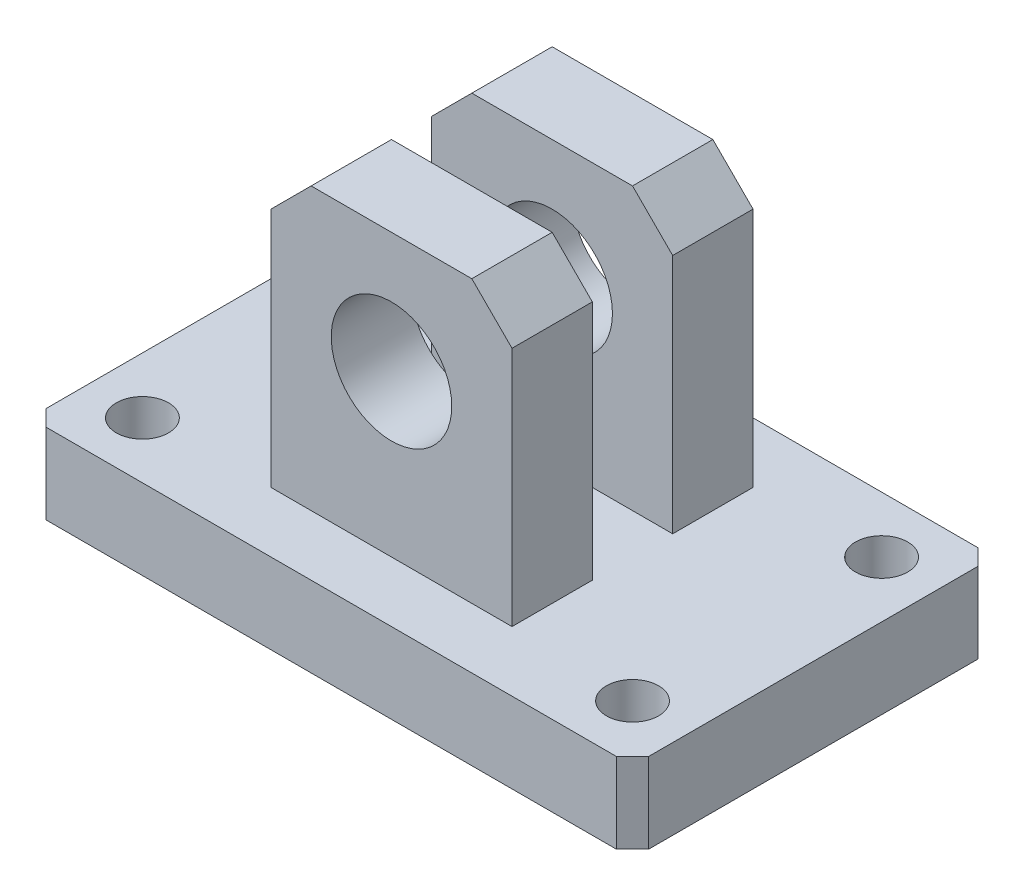
ISO-10303-21;
HEADER;
FILE_DESCRIPTION(('STEP AP214'),'2;1');
FILE_NAME('part.step','',(''),(''),'','','');
FILE_SCHEMA(('AUTOMOTIVE_DESIGN { 1 0 10303 214 1 1 1 1 }'));
ENDSEC;
DATA;
#1=APPLICATION_CONTEXT('core data for automotive mechanical design processes');
#2=APPLICATION_PROTOCOL_DEFINITION('international standard','automotive_design',2000,#1);
#3=PRODUCT_CONTEXT('',#1,'mechanical');
#4=PRODUCT('Part','Part','',(#3));
#5=PRODUCT_RELATED_PRODUCT_CATEGORY('part','',(#4));
#6=PRODUCT_DEFINITION_FORMATION('','',#4);
#7=PRODUCT_DEFINITION_CONTEXT('part definition',#1,'design');
#8=PRODUCT_DEFINITION('design','',#6,#7);
#9=PRODUCT_DEFINITION_SHAPE('','',#8);
#10=(LENGTH_UNIT() NAMED_UNIT(*) SI_UNIT(.MILLI.,.METRE.));
#11=(NAMED_UNIT(*) PLANE_ANGLE_UNIT() SI_UNIT($,.RADIAN.));
#12=(NAMED_UNIT(*) SI_UNIT($,.STERADIAN.) SOLID_ANGLE_UNIT());
#13=UNCERTAINTY_MEASURE_WITH_UNIT(LENGTH_MEASURE(1.E-05),#10,'distance_accuracy_value','');
#14=(GEOMETRIC_REPRESENTATION_CONTEXT(3) GLOBAL_UNCERTAINTY_ASSIGNED_CONTEXT((#13)) GLOBAL_UNIT_ASSIGNED_CONTEXT((#10,
#11,#12)) REPRESENTATION_CONTEXT('',''));
#15=CARTESIAN_POINT('',(0.,0.,0.));
#16=DIRECTION('',(0.,0.,1.));
#17=DIRECTION('',(1.,0.,0.));
#18=AXIS2_PLACEMENT_3D('',#15,#16,#17);
#19=CARTESIAN_POINT('',(0.,10.,0.));
#20=DIRECTION('',(0.,1.,0.));
#21=DIRECTION('',(0.,0.,1.));
#22=AXIS2_PLACEMENT_3D('',#19,#20,#21);
#23=PLANE('',#22);
#24=CARTESIAN_POINT('',(30.5,10.,-15.5));
#25=DIRECTION('',(0.,-1.,0.));
#26=DIRECTION('',(0.,0.,1.));
#27=AXIS2_PLACEMENT_3D('',#24,#25,#26);
#28=CIRCLE('',#27,3.25);
#29=CARTESIAN_POINT('',(30.5,10.,-12.25));
#30=VERTEX_POINT('',#29);
#31=EDGE_CURVE('E566',#30,#30,#28,.T.);
#32=ORIENTED_EDGE('',*,*,#31,.T.);
#33=EDGE_LOOP('',(#32));
#34=FACE_BOUND('',#33,.T.);
#35=CARTESIAN_POINT('',(30.5,10.,15.5));
#36=DIRECTION('',(0.,1.,0.));
#37=DIRECTION('',(0.,0.,-1.));
#38=AXIS2_PLACEMENT_3D('',#35,#36,#37);
#39=CIRCLE('',#38,3.25);
#40=CARTESIAN_POINT('',(30.5,10.,12.25));
#41=VERTEX_POINT('',#40);
#42=EDGE_CURVE('E576',#41,#41,#39,.T.);
#43=ORIENTED_EDGE('',*,*,#42,.F.);
#44=EDGE_LOOP('',(#43));
#45=FACE_BOUND('',#44,.T.);
#46=CARTESIAN_POINT('',(-30.5,10.,15.5));
#47=DIRECTION('',(0.,-1.,0.));
#48=DIRECTION('',(0.,0.,-1.));
#49=AXIS2_PLACEMENT_3D('',#46,#47,#48);
#50=CIRCLE('',#49,3.25);
#51=CARTESIAN_POINT('',(-30.5,10.,12.25));
#52=VERTEX_POINT('',#51);
#53=EDGE_CURVE('E581',#52,#52,#50,.T.);
#54=ORIENTED_EDGE('',*,*,#53,.T.);
#55=EDGE_LOOP('',(#54));
#56=FACE_BOUND('',#55,.T.);
#57=CARTESIAN_POINT('',(-30.5,10.,-15.5));
#58=DIRECTION('',(0.,1.,0.));
#59=DIRECTION('',(0.,0.,1.));
#60=AXIS2_PLACEMENT_3D('',#57,#58,#59);
#61=CIRCLE('',#60,3.25);
#62=CARTESIAN_POINT('',(-30.5,10.,-12.25));
#63=VERTEX_POINT('',#62);
#64=EDGE_CURVE('E589',#63,#63,#61,.T.);
#65=ORIENTED_EDGE('',*,*,#64,.F.);
#66=EDGE_LOOP('',(#65));
#67=FACE_BOUND('',#66,.T.);
#68=DIRECTION('',(0.,0.,1.));
#69=VECTOR('',#68,1.);
#70=CARTESIAN_POINT('',(15.,10.,-15.));
#71=LINE('',#70,#69);
#72=CARTESIAN_POINT('',(15.,10.,-15.));
#73=VERTEX_POINT('',#72);
#74=CARTESIAN_POINT('',(15.,10.,-5.00000000000001));
#75=VERTEX_POINT('',#74);
#76=EDGE_CURVE('E188',#73,#75,#71,.T.);
#77=ORIENTED_EDGE('',*,*,#76,.T.);
#78=DIRECTION('',(-1.,0.,0.));
#79=VECTOR('',#78,1.);
#80=CARTESIAN_POINT('',(-15.,10.,-5.00000000000001));
#81=LINE('',#80,#79);
#82=CARTESIAN_POINT('',(-15.,10.,-5.00000000000001));
#83=VERTEX_POINT('',#82);
#84=EDGE_CURVE('E196',#75,#83,#81,.T.);
#85=ORIENTED_EDGE('',*,*,#84,.T.);
#86=DIRECTION('',(0.,0.,-1.));
#87=VECTOR('',#86,1.);
#88=CARTESIAN_POINT('',(-15.,10.,-15.));
#89=LINE('',#88,#87);
#90=CARTESIAN_POINT('',(-15.,10.,-15.));
#91=VERTEX_POINT('',#90);
#92=EDGE_CURVE('E208',#83,#91,#89,.T.);
#93=ORIENTED_EDGE('',*,*,#92,.T.);
#94=DIRECTION('',(1.,0.,0.));
#95=VECTOR('',#94,1.);
#96=CARTESIAN_POINT('',(-15.,10.,-15.));
#97=LINE('',#96,#95);
#98=EDGE_CURVE('E203',#91,#73,#97,.T.);
#99=ORIENTED_EDGE('',*,*,#98,.T.);
#100=EDGE_LOOP('',(#77,#85,#93,#99));
#101=FACE_BOUND('',#100,.T.);
#102=DIRECTION('',(0.,0.,1.));
#103=VECTOR('',#102,1.);
#104=CARTESIAN_POINT('',(-37.5,10.,22.5));
#105=LINE('',#104,#103);
#106=CARTESIAN_POINT('',(-37.5,10.,-20.5));
#107=VERTEX_POINT('',#106);
#108=CARTESIAN_POINT('',(-37.5,10.,20.5));
#109=VERTEX_POINT('',#108);
#110=EDGE_CURVE('E250',#107,#109,#105,.T.);
#111=ORIENTED_EDGE('',*,*,#110,.T.);
#112=DIRECTION('',(-0.707106781186545,0.,-0.70710678118655));
#113=VECTOR('',#112,1.);
#114=CARTESIAN_POINT('',(-29.0000000000001,10.,28.9999999999999));
#115=LINE('',#114,#113);
#116=CARTESIAN_POINT('',(-35.5,10.,22.5));
#117=VERTEX_POINT('',#116);
#118=EDGE_CURVE('E322',#109,#117,#115,.F.);
#119=ORIENTED_EDGE('',*,*,#118,.T.);
#120=DIRECTION('',(1.,0.,0.));
#121=VECTOR('',#120,1.);
#122=CARTESIAN_POINT('',(37.5,10.,22.5));
#123=LINE('',#122,#121);
#124=CARTESIAN_POINT('',(35.5,10.,22.5));
#125=VERTEX_POINT('',#124);
#126=EDGE_CURVE('E247',#117,#125,#123,.T.);
#127=ORIENTED_EDGE('',*,*,#126,.T.);
#128=DIRECTION('',(-0.70710678118655,0.,0.707106781186545));
#129=VECTOR('',#128,1.);
#130=CARTESIAN_POINT('',(28.9999999999999,10.,29.0000000000001));
#131=LINE('',#130,#129);
#132=CARTESIAN_POINT('',(37.5,10.,20.5));
#133=VERTEX_POINT('',#132);
#134=EDGE_CURVE('E317',#125,#133,#131,.F.);
#135=ORIENTED_EDGE('',*,*,#134,.T.);
#136=DIRECTION('',(0.,0.,-1.));
#137=VECTOR('',#136,1.);
#138=CARTESIAN_POINT('',(37.5,10.,22.5));
#139=LINE('',#138,#137);
#140=CARTESIAN_POINT('',(37.5,10.,-20.5));
#141=VERTEX_POINT('',#140);
#142=EDGE_CURVE('E255',#133,#141,#139,.T.);
#143=ORIENTED_EDGE('',*,*,#142,.T.);
#144=DIRECTION('',(0.707106781186545,0.,0.70710678118655));
#145=VECTOR('',#144,1.);
#146=CARTESIAN_POINT('',(29.0000000000001,10.,-28.9999999999999));
#147=LINE('',#146,#145);
#148=CARTESIAN_POINT('',(35.5,10.,-22.5));
#149=VERTEX_POINT('',#148);
#150=EDGE_CURVE('E61',#141,#149,#147,.F.);
#151=ORIENTED_EDGE('',*,*,#150,.T.);
#152=DIRECTION('',(-1.,0.,0.));
#153=VECTOR('',#152,1.);
#154=CARTESIAN_POINT('',(37.5,10.,-22.5));
#155=LINE('',#154,#153);
#156=CARTESIAN_POINT('',(-35.5,10.,-22.5));
#157=VERTEX_POINT('',#156);
#158=EDGE_CURVE('E258',#149,#157,#155,.T.);
#159=ORIENTED_EDGE('',*,*,#158,.T.);
#160=DIRECTION('',(0.70710678118655,0.,-0.707106781186545));
#161=VECTOR('',#160,1.);
#162=CARTESIAN_POINT('',(-28.9999999999999,10.,-29.0000000000001));
#163=LINE('',#162,#161);
#164=EDGE_CURVE('E325',#157,#107,#163,.F.);
#165=ORIENTED_EDGE('',*,*,#164,.T.);
#166=EDGE_LOOP('',(#111,#119,#127,#135,#143,#151,#159,#165));
#167=FACE_BOUND('',#166,.T.);
#168=DIRECTION('',(-1.,0.,0.));
#169=VECTOR('',#168,1.);
#170=CARTESIAN_POINT('',(-15.,10.,5.00000000000001));
#171=LINE('',#170,#169);
#172=CARTESIAN_POINT('',(15.,10.,5.00000000000001));
#173=VERTEX_POINT('',#172);
#174=CARTESIAN_POINT('',(-15.,10.,5.00000000000001));
#175=VERTEX_POINT('',#174);
#176=EDGE_CURVE('E233',#173,#175,#171,.T.);
#177=ORIENTED_EDGE('',*,*,#176,.F.);
#178=DIRECTION('',(0.,0.,-1.));
#179=VECTOR('',#178,1.);
#180=CARTESIAN_POINT('',(15.,10.,15.));
#181=LINE('',#180,#179);
#182=CARTESIAN_POINT('',(15.,10.,15.));
#183=VERTEX_POINT('',#182);
#184=EDGE_CURVE('E219',#183,#173,#181,.T.);
#185=ORIENTED_EDGE('',*,*,#184,.F.);
#186=DIRECTION('',(1.,0.,0.));
#187=VECTOR('',#186,1.);
#188=CARTESIAN_POINT('',(-15.,10.,15.));
#189=LINE('',#188,#187);
#190=CARTESIAN_POINT('',(-15.,10.,15.));
#191=VERTEX_POINT('',#190);
#192=EDGE_CURVE('E223',#191,#183,#189,.T.);
#193=ORIENTED_EDGE('',*,*,#192,.F.);
#194=DIRECTION('',(0.,0.,1.));
#195=VECTOR('',#194,1.);
#196=CARTESIAN_POINT('',(-15.,10.,15.));
#197=LINE('',#196,#195);
#198=EDGE_CURVE('E234',#175,#191,#197,.T.);
#199=ORIENTED_EDGE('',*,*,#198,.F.);
#200=EDGE_LOOP('',(#177,#185,#193,#199));
#201=FACE_BOUND('',#200,.T.);
#202=ADVANCED_FACE('F41',(#34,#45,#56,#67,#101,#167,#201),#23,.T.);
#203=CARTESIAN_POINT('',(-37.5,10.,22.5));
#204=DIRECTION('',(1.,0.,0.));
#205=DIRECTION('',(0.,0.,-1.));
#206=AXIS2_PLACEMENT_3D('',#203,#204,#205);
#207=PLANE('',#206);
#208=DIRECTION('',(0.,0.,1.));
#209=VECTOR('',#208,1.);
#210=CARTESIAN_POINT('',(-37.5,0.,22.5));
#211=LINE('',#210,#209);
#212=CARTESIAN_POINT('',(-37.5,0.,-20.5));
#213=VERTEX_POINT('',#212);
#214=CARTESIAN_POINT('',(-37.5,0.,20.5));
#215=VERTEX_POINT('',#214);
#216=EDGE_CURVE('E248',#213,#215,#211,.T.);
#217=ORIENTED_EDGE('',*,*,#216,.T.);
#218=DIRECTION('',(0.,1.,0.));
#219=VECTOR('',#218,1.);
#220=CARTESIAN_POINT('',(-37.5,10.,20.5));
#221=LINE('',#220,#219);
#222=EDGE_CURVE('E320',#215,#109,#221,.T.);
#223=ORIENTED_EDGE('',*,*,#222,.T.);
#224=ORIENTED_EDGE('',*,*,#110,.F.);
#225=DIRECTION('',(0.,-1.,0.));
#226=VECTOR('',#225,1.);
#227=CARTESIAN_POINT('',(-37.5,10.,-20.5));
#228=LINE('',#227,#226);
#229=EDGE_CURVE('E314',#107,#213,#228,.T.);
#230=ORIENTED_EDGE('',*,*,#229,.T.);
#231=EDGE_LOOP('',(#217,#223,#224,#230));
#232=FACE_BOUND('',#231,.T.);
#233=ADVANCED_FACE('F351',(#232),#207,.F.);
#234=CARTESIAN_POINT('',(37.5,10.,22.5));
#235=DIRECTION('',(0.,0.,-1.));
#236=DIRECTION('',(-1.,0.,0.));
#237=AXIS2_PLACEMENT_3D('',#234,#235,#236);
#238=PLANE('',#237);
#239=ORIENTED_EDGE('',*,*,#126,.F.);
#240=DIRECTION('',(0.,-1.,0.));
#241=VECTOR('',#240,1.);
#242=CARTESIAN_POINT('',(-35.5,10.,22.5));
#243=LINE('',#242,#241);
#244=CARTESIAN_POINT('',(-35.5,0.,22.5));
#245=VERTEX_POINT('',#244);
#246=EDGE_CURVE('E301',#117,#245,#243,.T.);
#247=ORIENTED_EDGE('',*,*,#246,.T.);
#248=DIRECTION('',(1.,0.,0.));
#249=VECTOR('',#248,1.);
#250=CARTESIAN_POINT('',(37.5,0.,22.5));
#251=LINE('',#250,#249);
#252=CARTESIAN_POINT('',(35.5,0.,22.5));
#253=VERTEX_POINT('',#252);
#254=EDGE_CURVE('E261',#245,#253,#251,.T.);
#255=ORIENTED_EDGE('',*,*,#254,.T.);
#256=DIRECTION('',(0.,1.,0.));
#257=VECTOR('',#256,1.);
#258=CARTESIAN_POINT('',(35.5,10.,22.5));
#259=LINE('',#258,#257);
#260=EDGE_CURVE('E303',#253,#125,#259,.T.);
#261=ORIENTED_EDGE('',*,*,#260,.T.);
#262=EDGE_LOOP('',(#239,#247,#255,#261));
#263=FACE_BOUND('',#262,.T.);
#264=ADVANCED_FACE('F361',(#263),#238,.F.);
#265=CARTESIAN_POINT('',(37.5,10.,22.5));
#266=DIRECTION('',(-1.,0.,0.));
#267=DIRECTION('',(0.,0.,1.));
#268=AXIS2_PLACEMENT_3D('',#265,#266,#267);
#269=PLANE('',#268);
#270=DIRECTION('',(0.,0.,-1.));
#271=VECTOR('',#270,1.);
#272=CARTESIAN_POINT('',(37.5,0.,22.5));
#273=LINE('',#272,#271);
#274=CARTESIAN_POINT('',(37.5,0.,20.5));
#275=VERTEX_POINT('',#274);
#276=CARTESIAN_POINT('',(37.5,0.,-20.5));
#277=VERTEX_POINT('',#276);
#278=EDGE_CURVE('E262',#275,#277,#273,.T.);
#279=ORIENTED_EDGE('',*,*,#278,.T.);
#280=DIRECTION('',(0.,1.,0.));
#281=VECTOR('',#280,1.);
#282=CARTESIAN_POINT('',(37.5,10.,-20.5));
#283=LINE('',#282,#281);
#284=EDGE_CURVE('E11',#277,#141,#283,.T.);
#285=ORIENTED_EDGE('',*,*,#284,.T.);
#286=ORIENTED_EDGE('',*,*,#142,.F.);
#287=DIRECTION('',(0.,-1.,0.));
#288=VECTOR('',#287,1.);
#289=CARTESIAN_POINT('',(37.5,10.,20.5));
#290=LINE('',#289,#288);
#291=EDGE_CURVE('E51',#133,#275,#290,.T.);
#292=ORIENTED_EDGE('',*,*,#291,.T.);
#293=EDGE_LOOP('',(#279,#285,#286,#292));
#294=FACE_BOUND('',#293,.T.);
#295=ADVANCED_FACE('F333',(#294),#269,.F.);
#296=CARTESIAN_POINT('',(37.5,10.,-22.5));
#297=DIRECTION('',(0.,0.,1.));
#298=DIRECTION('',(1.,0.,0.));
#299=AXIS2_PLACEMENT_3D('',#296,#297,#298);
#300=PLANE('',#299);
#301=DIRECTION('',(-1.,0.,0.));
#302=VECTOR('',#301,1.);
#303=CARTESIAN_POINT('',(37.5,0.,-22.5));
#304=LINE('',#303,#302);
#305=CARTESIAN_POINT('',(35.5,0.,-22.5));
#306=VERTEX_POINT('',#305);
#307=CARTESIAN_POINT('',(-35.5,0.,-22.5));
#308=VERTEX_POINT('',#307);
#309=EDGE_CURVE('E253',#306,#308,#304,.T.);
#310=ORIENTED_EDGE('',*,*,#309,.T.);
#311=DIRECTION('',(0.,1.,0.));
#312=VECTOR('',#311,1.);
#313=CARTESIAN_POINT('',(-35.5,10.,-22.5));
#314=LINE('',#313,#312);
#315=EDGE_CURVE('E59',#308,#157,#314,.T.);
#316=ORIENTED_EDGE('',*,*,#315,.T.);
#317=ORIENTED_EDGE('',*,*,#158,.F.);
#318=DIRECTION('',(0.,-1.,0.));
#319=VECTOR('',#318,1.);
#320=CARTESIAN_POINT('',(35.5,10.,-22.5));
#321=LINE('',#320,#319);
#322=EDGE_CURVE('E326',#149,#306,#321,.T.);
#323=ORIENTED_EDGE('',*,*,#322,.T.);
#324=EDGE_LOOP('',(#310,#316,#317,#323));
#325=FACE_BOUND('',#324,.T.);
#326=ADVANCED_FACE('F347',(#325),#300,.F.);
#327=CARTESIAN_POINT('',(0.,0.,0.));
#328=DIRECTION('',(0.,1.,0.));
#329=DIRECTION('',(0.,0.,1.));
#330=AXIS2_PLACEMENT_3D('',#327,#328,#329);
#331=PLANE('',#330);
#332=CARTESIAN_POINT('',(30.5,0.,-15.5));
#333=DIRECTION('',(0.,-1.,0.));
#334=DIRECTION('',(0.,0.,1.));
#335=AXIS2_PLACEMENT_3D('',#332,#333,#334);
#336=CIRCLE('',#335,3.25);
#337=CARTESIAN_POINT('',(30.5,0.,-12.25));
#338=VERTEX_POINT('',#337);
#339=EDGE_CURVE('E573',#338,#338,#336,.T.);
#340=ORIENTED_EDGE('',*,*,#339,.F.);
#341=EDGE_LOOP('',(#340));
#342=FACE_BOUND('',#341,.T.);
#343=CARTESIAN_POINT('',(30.5,0.,15.5));
#344=DIRECTION('',(0.,1.,0.));
#345=DIRECTION('',(0.,0.,-1.));
#346=AXIS2_PLACEMENT_3D('',#343,#344,#345);
#347=CIRCLE('',#346,3.25);
#348=CARTESIAN_POINT('',(30.5,0.,12.25));
#349=VERTEX_POINT('',#348);
#350=EDGE_CURVE('E577',#349,#349,#347,.T.);
#351=ORIENTED_EDGE('',*,*,#350,.T.);
#352=EDGE_LOOP('',(#351));
#353=FACE_BOUND('',#352,.T.);
#354=CARTESIAN_POINT('',(-30.5,0.,15.5));
#355=DIRECTION('',(0.,-1.,0.));
#356=DIRECTION('',(0.,0.,-1.));
#357=AXIS2_PLACEMENT_3D('',#354,#355,#356);
#358=CIRCLE('',#357,3.25);
#359=CARTESIAN_POINT('',(-30.5,0.,12.25));
#360=VERTEX_POINT('',#359);
#361=EDGE_CURVE('E588',#360,#360,#358,.T.);
#362=ORIENTED_EDGE('',*,*,#361,.F.);
#363=EDGE_LOOP('',(#362));
#364=FACE_BOUND('',#363,.T.);
#365=CARTESIAN_POINT('',(-30.5,0.,-15.5));
#366=DIRECTION('',(0.,1.,0.));
#367=DIRECTION('',(0.,0.,1.));
#368=AXIS2_PLACEMENT_3D('',#365,#366,#367);
#369=CIRCLE('',#368,3.25);
#370=CARTESIAN_POINT('',(-30.5,0.,-12.25));
#371=VERTEX_POINT('',#370);
#372=EDGE_CURVE('E205',#371,#371,#369,.T.);
#373=ORIENTED_EDGE('',*,*,#372,.T.);
#374=EDGE_LOOP('',(#373));
#375=FACE_BOUND('',#374,.T.);
#376=ORIENTED_EDGE('',*,*,#254,.F.);
#377=DIRECTION('',(0.707106781186545,0.,0.70710678118655));
#378=VECTOR('',#377,1.);
#379=CARTESIAN_POINT('',(-35.5,0.,22.5));
#380=LINE('',#379,#378);
#381=EDGE_CURVE('E315',#245,#215,#380,.F.);
#382=ORIENTED_EDGE('',*,*,#381,.T.);
#383=ORIENTED_EDGE('',*,*,#216,.F.);
#384=DIRECTION('',(-0.70710678118655,0.,0.707106781186545));
#385=VECTOR('',#384,1.);
#386=CARTESIAN_POINT('',(-37.5,0.,-20.5));
#387=LINE('',#386,#385);
#388=EDGE_CURVE('E309',#213,#308,#387,.F.);
#389=ORIENTED_EDGE('',*,*,#388,.T.);
#390=ORIENTED_EDGE('',*,*,#309,.F.);
#391=DIRECTION('',(-0.707106781186545,0.,-0.70710678118655));
#392=VECTOR('',#391,1.);
#393=CARTESIAN_POINT('',(35.5,0.,-22.5));
#394=LINE('',#393,#392);
#395=EDGE_CURVE('E306',#306,#277,#394,.F.);
#396=ORIENTED_EDGE('',*,*,#395,.T.);
#397=ORIENTED_EDGE('',*,*,#278,.F.);
#398=DIRECTION('',(0.70710678118655,0.,-0.707106781186545));
#399=VECTOR('',#398,1.);
#400=CARTESIAN_POINT('',(37.5,0.,20.5));
#401=LINE('',#400,#399);
#402=EDGE_CURVE('E308',#275,#253,#401,.F.);
#403=ORIENTED_EDGE('',*,*,#402,.T.);
#404=EDGE_LOOP('',(#376,#382,#383,#389,#390,#396,#397,#403));
#405=FACE_BOUND('',#404,.T.);
#406=ADVANCED_FACE('F343',(#342,#353,#364,#375,#405),#331,.F.);
#407=CARTESIAN_POINT('',(15.,45.,15.));
#408=DIRECTION('',(-1.,0.,0.));
#409=DIRECTION('',(0.,0.,1.));
#410=AXIS2_PLACEMENT_3D('',#407,#408,#409);
#411=PLANE('',#410);
#412=DIRECTION('',(0.,-1.,0.));
#413=VECTOR('',#412,1.);
#414=CARTESIAN_POINT('',(15.,45.,5.00000000000001));
#415=LINE('',#414,#413);
#416=CARTESIAN_POINT('',(15.,40.,5.00000000000001));
#417=VERTEX_POINT('',#416);
#418=EDGE_CURVE('E245',#417,#173,#415,.T.);
#419=ORIENTED_EDGE('',*,*,#418,.F.);
#420=DIRECTION('',(0.,0.,1.));
#421=VECTOR('',#420,1.);
#422=CARTESIAN_POINT('',(15.,40.,15.));
#423=LINE('',#422,#421);
#424=CARTESIAN_POINT('',(15.,40.,15.));
#425=VERTEX_POINT('',#424);
#426=EDGE_CURVE('E300',#417,#425,#423,.T.);
#427=ORIENTED_EDGE('',*,*,#426,.T.);
#428=DIRECTION('',(0.,-1.,0.));
#429=VECTOR('',#428,1.);
#430=CARTESIAN_POINT('',(15.,45.,15.));
#431=LINE('',#430,#429);
#432=EDGE_CURVE('E227',#425,#183,#431,.T.);
#433=ORIENTED_EDGE('',*,*,#432,.T.);
#434=ORIENTED_EDGE('',*,*,#184,.T.);
#435=EDGE_LOOP('',(#419,#427,#433,#434));
#436=FACE_BOUND('',#435,.T.);
#437=ADVANCED_FACE('F390',(#436),#411,.F.);
#438=CARTESIAN_POINT('',(-15.,45.,5.00000000000001));
#439=DIRECTION('',(0.,0.,1.));
#440=DIRECTION('',(1.,0.,0.));
#441=AXIS2_PLACEMENT_3D('',#438,#439,#440);
#442=PLANE('',#441);
#443=CARTESIAN_POINT('',(0.,30.,5.00000000000001));
#444=DIRECTION('',(0.,0.,1.));
#445=DIRECTION('',(1.,0.,0.));
#446=AXIS2_PLACEMENT_3D('',#443,#444,#445);
#447=CIRCLE('',#446,7.5);
#448=CARTESIAN_POINT('',(7.5,30.,5.00000000000001));
#449=VERTEX_POINT('',#448);
#450=EDGE_CURVE('E549',#449,#449,#447,.T.);
#451=ORIENTED_EDGE('',*,*,#450,.T.);
#452=EDGE_LOOP('',(#451));
#453=FACE_BOUND('',#452,.T.);
#454=DIRECTION('',(0.,-1.,0.));
#455=VECTOR('',#454,1.);
#456=CARTESIAN_POINT('',(-15.,45.,5.00000000000001));
#457=LINE('',#456,#455);
#458=CARTESIAN_POINT('',(-15.,40.,5.00000000000001));
#459=VERTEX_POINT('',#458);
#460=EDGE_CURVE('E244',#459,#175,#457,.T.);
#461=ORIENTED_EDGE('',*,*,#460,.F.);
#462=DIRECTION('',(-0.707106781186547,-0.707106781186549,0.));
#463=VECTOR('',#462,1.);
#464=CARTESIAN_POINT('',(-9.99999999999999,45.,5.00000000000001));
#465=LINE('',#464,#463);
#466=CARTESIAN_POINT('',(-9.99999999999999,45.,5.00000000000001));
#467=VERTEX_POINT('',#466);
#468=EDGE_CURVE('E283',#459,#467,#465,.F.);
#469=ORIENTED_EDGE('',*,*,#468,.T.);
#470=DIRECTION('',(-1.,0.,0.));
#471=VECTOR('',#470,1.);
#472=CARTESIAN_POINT('',(-15.,45.,5.00000000000001));
#473=LINE('',#472,#471);
#474=CARTESIAN_POINT('',(10.,45.,5.00000000000001));
#475=VERTEX_POINT('',#474);
#476=EDGE_CURVE('E222',#475,#467,#473,.T.);
#477=ORIENTED_EDGE('',*,*,#476,.F.);
#478=DIRECTION('',(-0.707106781186547,0.707106781186549,0.));
#479=VECTOR('',#478,1.);
#480=CARTESIAN_POINT('',(10.,45.,5.00000000000001));
#481=LINE('',#480,#479);
#482=EDGE_CURVE('E276',#475,#417,#481,.F.);
#483=ORIENTED_EDGE('',*,*,#482,.T.);
#484=ORIENTED_EDGE('',*,*,#418,.T.);
#485=ORIENTED_EDGE('',*,*,#176,.T.);
#486=EDGE_LOOP('',(#461,#469,#477,#483,#484,#485));
#487=FACE_BOUND('',#486,.T.);
#488=ADVANCED_FACE('F539',(#453,#487),#442,.F.);
#489=CARTESIAN_POINT('',(-15.,45.,15.));
#490=DIRECTION('',(1.,0.,0.));
#491=DIRECTION('',(0.,0.,-1.));
#492=AXIS2_PLACEMENT_3D('',#489,#490,#491);
#493=PLANE('',#492);
#494=DIRECTION('',(0.,-1.,0.));
#495=VECTOR('',#494,1.);
#496=CARTESIAN_POINT('',(-15.,45.,15.));
#497=LINE('',#496,#495);
#498=CARTESIAN_POINT('',(-15.,40.,15.));
#499=VERTEX_POINT('',#498);
#500=EDGE_CURVE('E238',#499,#191,#497,.T.);
#501=ORIENTED_EDGE('',*,*,#500,.F.);
#502=DIRECTION('',(0.,0.,-1.));
#503=VECTOR('',#502,1.);
#504=CARTESIAN_POINT('',(-15.,40.,15.));
#505=LINE('',#504,#503);
#506=EDGE_CURVE('E280',#499,#459,#505,.T.);
#507=ORIENTED_EDGE('',*,*,#506,.T.);
#508=ORIENTED_EDGE('',*,*,#460,.T.);
#509=ORIENTED_EDGE('',*,*,#198,.T.);
#510=EDGE_LOOP('',(#501,#507,#508,#509));
#511=FACE_BOUND('',#510,.T.);
#512=ADVANCED_FACE('F540',(#511),#493,.F.);
#513=CARTESIAN_POINT('',(-15.,45.,15.));
#514=DIRECTION('',(0.,0.,-1.));
#515=DIRECTION('',(-1.,0.,0.));
#516=AXIS2_PLACEMENT_3D('',#513,#514,#515);
#517=PLANE('',#516);
#518=CARTESIAN_POINT('',(0.,30.,15.));
#519=DIRECTION('',(0.,0.,1.));
#520=DIRECTION('',(1.,0.,0.));
#521=AXIS2_PLACEMENT_3D('',#518,#519,#520);
#522=CIRCLE('',#521,7.5);
#523=CARTESIAN_POINT('',(7.5,30.,15.));
#524=VERTEX_POINT('',#523);
#525=EDGE_CURVE('E625',#524,#524,#522,.T.);
#526=ORIENTED_EDGE('',*,*,#525,.F.);
#527=EDGE_LOOP('',(#526));
#528=FACE_BOUND('',#527,.T.);
#529=DIRECTION('',(1.,0.,0.));
#530=VECTOR('',#529,1.);
#531=CARTESIAN_POINT('',(-15.,45.,15.));
#532=LINE('',#531,#530);
#533=CARTESIAN_POINT('',(-9.99999999999999,45.,15.));
#534=VERTEX_POINT('',#533);
#535=CARTESIAN_POINT('',(10.,45.,15.));
#536=VERTEX_POINT('',#535);
#537=EDGE_CURVE('E221',#534,#536,#532,.T.);
#538=ORIENTED_EDGE('',*,*,#537,.F.);
#539=DIRECTION('',(0.707106781186547,0.707106781186549,0.));
#540=VECTOR('',#539,1.);
#541=CARTESIAN_POINT('',(-9.99999999999999,45.,15.));
#542=LINE('',#541,#540);
#543=EDGE_CURVE('E274',#534,#499,#542,.F.);
#544=ORIENTED_EDGE('',*,*,#543,.T.);
#545=ORIENTED_EDGE('',*,*,#500,.T.);
#546=ORIENTED_EDGE('',*,*,#192,.T.);
#547=ORIENTED_EDGE('',*,*,#432,.F.);
#548=DIRECTION('',(0.707106781186547,-0.707106781186549,0.));
#549=VECTOR('',#548,1.);
#550=CARTESIAN_POINT('',(10.,45.,15.));
#551=LINE('',#550,#549);
#552=EDGE_CURVE('E272',#425,#536,#551,.F.);
#553=ORIENTED_EDGE('',*,*,#552,.T.);
#554=EDGE_LOOP('',(#538,#544,#545,#546,#547,#553));
#555=FACE_BOUND('',#554,.T.);
#556=ADVANCED_FACE('F531',(#528,#555),#517,.F.);
#557=CARTESIAN_POINT('',(0.,45.,0.));
#558=DIRECTION('',(0.,-1.,0.));
#559=DIRECTION('',(0.,0.,-1.));
#560=AXIS2_PLACEMENT_3D('',#557,#558,#559);
#561=PLANE('',#560);
#562=ORIENTED_EDGE('',*,*,#476,.T.);
#563=DIRECTION('',(0.,0.,1.));
#564=VECTOR('',#563,1.);
#565=CARTESIAN_POINT('',(-9.99999999999999,45.,0.));
#566=LINE('',#565,#564);
#567=EDGE_CURVE('E269',#467,#534,#566,.T.);
#568=ORIENTED_EDGE('',*,*,#567,.T.);
#569=ORIENTED_EDGE('',*,*,#537,.T.);
#570=DIRECTION('',(0.,0.,-1.));
#571=VECTOR('',#570,1.);
#572=CARTESIAN_POINT('',(10.,45.,0.));
#573=LINE('',#572,#571);
#574=EDGE_CURVE('E256',#536,#475,#573,.T.);
#575=ORIENTED_EDGE('',*,*,#574,.T.);
#576=EDGE_LOOP('',(#562,#568,#569,#575));
#577=FACE_BOUND('',#576,.T.);
#578=ADVANCED_FACE('F529',(#577),#561,.F.);
#579=CARTESIAN_POINT('',(15.,45.,-15.));
#580=DIRECTION('',(1.,0.,0.));
#581=DIRECTION('',(0.,0.,-1.));
#582=AXIS2_PLACEMENT_3D('',#579,#580,#581);
#583=PLANE('',#582);
#584=DIRECTION('',(0.,-1.,0.));
#585=VECTOR('',#584,1.);
#586=CARTESIAN_POINT('',(15.,45.,-15.));
#587=LINE('',#586,#585);
#588=CARTESIAN_POINT('',(15.,40.,-15.));
#589=VERTEX_POINT('',#588);
#590=EDGE_CURVE('E217',#589,#73,#587,.T.);
#591=ORIENTED_EDGE('',*,*,#590,.F.);
#592=DIRECTION('',(0.,0.,1.));
#593=VECTOR('',#592,1.);
#594=CARTESIAN_POINT('',(15.,40.,-5.00000000000001));
#595=LINE('',#594,#593);
#596=CARTESIAN_POINT('',(15.,40.,-5.00000000000001));
#597=VERTEX_POINT('',#596);
#598=EDGE_CURVE('E187',#589,#597,#595,.T.);
#599=ORIENTED_EDGE('',*,*,#598,.T.);
#600=DIRECTION('',(0.,-1.,0.));
#601=VECTOR('',#600,1.);
#602=CARTESIAN_POINT('',(15.,45.,-5.00000000000001));
#603=LINE('',#602,#601);
#604=EDGE_CURVE('E185',#597,#75,#603,.T.);
#605=ORIENTED_EDGE('',*,*,#604,.T.);
#606=ORIENTED_EDGE('',*,*,#76,.F.);
#607=EDGE_LOOP('',(#591,#599,#605,#606));
#608=FACE_BOUND('',#607,.T.);
#609=ADVANCED_FACE('F183',(#608),#583,.T.);
#610=CARTESIAN_POINT('',(-15.,45.,-15.));
#611=DIRECTION('',(0.,0.,-1.));
#612=DIRECTION('',(-1.,0.,0.));
#613=AXIS2_PLACEMENT_3D('',#610,#611,#612);
#614=PLANE('',#613);
#615=CARTESIAN_POINT('',(0.,30.,-15.));
#616=DIRECTION('',(0.,0.,-1.));
#617=DIRECTION('',(-1.,0.,0.));
#618=AXIS2_PLACEMENT_3D('',#615,#616,#617);
#619=CIRCLE('',#618,7.5);
#620=CARTESIAN_POINT('',(-7.5,30.,-15.));
#621=VERTEX_POINT('',#620);
#622=EDGE_CURVE('E569',#621,#621,#619,.T.);
#623=ORIENTED_EDGE('',*,*,#622,.F.);
#624=EDGE_LOOP('',(#623));
#625=FACE_BOUND('',#624,.T.);
#626=DIRECTION('',(0.,-1.,0.));
#627=VECTOR('',#626,1.);
#628=CARTESIAN_POINT('',(-15.,45.,-15.));
#629=LINE('',#628,#627);
#630=CARTESIAN_POINT('',(-15.,40.,-15.));
#631=VERTEX_POINT('',#630);
#632=EDGE_CURVE('E216',#631,#91,#629,.T.);
#633=ORIENTED_EDGE('',*,*,#632,.F.);
#634=DIRECTION('',(0.707106781186549,0.707106781186546,0.));
#635=VECTOR('',#634,1.);
#636=CARTESIAN_POINT('',(-12.5,42.5,-15.));
#637=LINE('',#636,#635);
#638=CARTESIAN_POINT('',(-9.99999999999997,45.,-15.));
#639=VERTEX_POINT('',#638);
#640=EDGE_CURVE('E286',#631,#639,#637,.T.);
#641=ORIENTED_EDGE('',*,*,#640,.T.);
#642=DIRECTION('',(1.,0.,0.));
#643=VECTOR('',#642,1.);
#644=CARTESIAN_POINT('',(-15.,45.,-15.));
#645=LINE('',#644,#643);
#646=CARTESIAN_POINT('',(9.99999999999997,45.,-15.));
#647=VERTEX_POINT('',#646);
#648=EDGE_CURVE('E210',#639,#647,#645,.T.);
#649=ORIENTED_EDGE('',*,*,#648,.T.);
#650=DIRECTION('',(0.707106781186549,-0.707106781186546,0.));
#651=VECTOR('',#650,1.);
#652=CARTESIAN_POINT('',(-2.50000000000008,57.5,-15.));
#653=LINE('',#652,#651);
#654=EDGE_CURVE('E288',#647,#589,#653,.T.);
#655=ORIENTED_EDGE('',*,*,#654,.T.);
#656=ORIENTED_EDGE('',*,*,#590,.T.);
#657=ORIENTED_EDGE('',*,*,#98,.F.);
#658=EDGE_LOOP('',(#633,#641,#649,#655,#656,#657));
#659=FACE_BOUND('',#658,.T.);
#660=ADVANCED_FACE('F521',(#625,#659),#614,.T.);
#661=CARTESIAN_POINT('',(-15.,45.,-15.));
#662=DIRECTION('',(-1.,0.,0.));
#663=DIRECTION('',(0.,0.,1.));
#664=AXIS2_PLACEMENT_3D('',#661,#662,#663);
#665=PLANE('',#664);
#666=DIRECTION('',(0.,-1.,0.));
#667=VECTOR('',#666,1.);
#668=CARTESIAN_POINT('',(-15.,45.,-5.00000000000001));
#669=LINE('',#668,#667);
#670=CARTESIAN_POINT('',(-15.,40.,-5.00000000000001));
#671=VERTEX_POINT('',#670);
#672=EDGE_CURVE('E193',#671,#83,#669,.T.);
#673=ORIENTED_EDGE('',*,*,#672,.F.);
#674=DIRECTION('',(0.,0.,-1.));
#675=VECTOR('',#674,1.);
#676=CARTESIAN_POINT('',(-15.,40.,-15.));
#677=LINE('',#676,#675);
#678=EDGE_CURVE('E282',#671,#631,#677,.T.);
#679=ORIENTED_EDGE('',*,*,#678,.T.);
#680=ORIENTED_EDGE('',*,*,#632,.T.);
#681=ORIENTED_EDGE('',*,*,#92,.F.);
#682=EDGE_LOOP('',(#673,#679,#680,#681));
#683=FACE_BOUND('',#682,.T.);
#684=ADVANCED_FACE('F520',(#683),#665,.T.);
#685=CARTESIAN_POINT('',(-15.,45.,-5.00000000000001));
#686=DIRECTION('',(0.,0.,1.));
#687=DIRECTION('',(1.,0.,0.));
#688=AXIS2_PLACEMENT_3D('',#685,#686,#687);
#689=PLANE('',#688);
#690=CARTESIAN_POINT('',(0.,30.,-5.00000000000001));
#691=DIRECTION('',(0.,0.,1.));
#692=DIRECTION('',(1.,0.,0.));
#693=AXIS2_PLACEMENT_3D('',#690,#691,#692);
#694=CIRCLE('',#693,7.5);
#695=CARTESIAN_POINT('',(7.5,30.,-5.00000000000001));
#696=VERTEX_POINT('',#695);
#697=EDGE_CURVE('E46',#696,#696,#694,.T.);
#698=ORIENTED_EDGE('',*,*,#697,.F.);
#699=EDGE_LOOP('',(#698));
#700=FACE_BOUND('',#699,.T.);
#701=DIRECTION('',(-1.,0.,0.));
#702=VECTOR('',#701,1.);
#703=CARTESIAN_POINT('',(-15.,45.,-5.00000000000001));
#704=LINE('',#703,#702);
#705=CARTESIAN_POINT('',(9.99999999999997,45.,-5.00000000000001));
#706=VERTEX_POINT('',#705);
#707=CARTESIAN_POINT('',(-9.99999999999997,45.,-5.00000000000001));
#708=VERTEX_POINT('',#707);
#709=EDGE_CURVE('E195',#706,#708,#704,.T.);
#710=ORIENTED_EDGE('',*,*,#709,.T.);
#711=DIRECTION('',(-0.707106781186549,-0.707106781186546,0.));
#712=VECTOR('',#711,1.);
#713=CARTESIAN_POINT('',(-12.5,42.5,-5.00000000000001));
#714=LINE('',#713,#712);
#715=EDGE_CURVE('E298',#708,#671,#714,.T.);
#716=ORIENTED_EDGE('',*,*,#715,.T.);
#717=ORIENTED_EDGE('',*,*,#672,.T.);
#718=ORIENTED_EDGE('',*,*,#84,.F.);
#719=ORIENTED_EDGE('',*,*,#604,.F.);
#720=DIRECTION('',(-0.707106781186549,0.707106781186546,0.));
#721=VECTOR('',#720,1.);
#722=CARTESIAN_POINT('',(-2.50000000000008,57.5,-5.00000000000001));
#723=LINE('',#722,#721);
#724=EDGE_CURVE('E294',#597,#706,#723,.T.);
#725=ORIENTED_EDGE('',*,*,#724,.T.);
#726=EDGE_LOOP('',(#710,#716,#717,#718,#719,#725));
#727=FACE_BOUND('',#726,.T.);
#728=ADVANCED_FACE('F202',(#700,#727),#689,.T.);
#729=CARTESIAN_POINT('',(0.,45.,0.));
#730=DIRECTION('',(0.,-1.,0.));
#731=DIRECTION('',(0.,0.,1.));
#732=AXIS2_PLACEMENT_3D('',#729,#730,#731);
#733=PLANE('',#732);
#734=ORIENTED_EDGE('',*,*,#648,.F.);
#735=DIRECTION('',(0.,0.,1.));
#736=VECTOR('',#735,1.);
#737=CARTESIAN_POINT('',(-9.99999999999997,45.,-5.00000000000001));
#738=LINE('',#737,#736);
#739=EDGE_CURVE('E295',#639,#708,#738,.T.);
#740=ORIENTED_EDGE('',*,*,#739,.T.);
#741=ORIENTED_EDGE('',*,*,#709,.F.);
#742=DIRECTION('',(0.,0.,-1.));
#743=VECTOR('',#742,1.);
#744=CARTESIAN_POINT('',(9.99999999999997,45.,-15.));
#745=LINE('',#744,#743);
#746=EDGE_CURVE('E287',#706,#647,#745,.T.);
#747=ORIENTED_EDGE('',*,*,#746,.T.);
#748=EDGE_LOOP('',(#734,#740,#741,#747));
#749=FACE_BOUND('',#748,.T.);
#750=ADVANCED_FACE('F403',(#749),#733,.F.);
#751=CARTESIAN_POINT('',(-9.99999999999999,45.,0.));
#752=DIRECTION('',(0.707106781186549,-0.707106781186547,0.));
#753=DIRECTION('',(0.,0.,1.));
#754=AXIS2_PLACEMENT_3D('',#751,#752,#753);
#755=PLANE('',#754);
#756=ORIENTED_EDGE('',*,*,#468,.F.);
#757=ORIENTED_EDGE('',*,*,#506,.F.);
#758=ORIENTED_EDGE('',*,*,#543,.F.);
#759=ORIENTED_EDGE('',*,*,#567,.F.);
#760=EDGE_LOOP('',(#756,#757,#758,#759));
#761=FACE_BOUND('',#760,.T.);
#762=ADVANCED_FACE('F396',(#761),#755,.F.);
#763=CARTESIAN_POINT('',(-15.,40.,-15.));
#764=DIRECTION('',(-0.707106781186545,0.707106781186549,0.));
#765=DIRECTION('',(0.,0.,1.));
#766=AXIS2_PLACEMENT_3D('',#763,#764,#765);
#767=PLANE('',#766);
#768=ORIENTED_EDGE('',*,*,#715,.F.);
#769=ORIENTED_EDGE('',*,*,#739,.F.);
#770=ORIENTED_EDGE('',*,*,#640,.F.);
#771=ORIENTED_EDGE('',*,*,#678,.F.);
#772=EDGE_LOOP('',(#768,#769,#770,#771));
#773=FACE_BOUND('',#772,.T.);
#774=ADVANCED_FACE('F404',(#773),#767,.T.);
#775=CARTESIAN_POINT('',(15.,40.,-15.));
#776=DIRECTION('',(0.707106781186545,0.707106781186549,0.));
#777=DIRECTION('',(0.,0.,-1.));
#778=AXIS2_PLACEMENT_3D('',#775,#776,#777);
#779=PLANE('',#778);
#780=ORIENTED_EDGE('',*,*,#654,.F.);
#781=ORIENTED_EDGE('',*,*,#746,.F.);
#782=ORIENTED_EDGE('',*,*,#724,.F.);
#783=ORIENTED_EDGE('',*,*,#598,.F.);
#784=EDGE_LOOP('',(#780,#781,#782,#783));
#785=FACE_BOUND('',#784,.T.);
#786=ADVANCED_FACE('F415',(#785),#779,.T.);
#787=CARTESIAN_POINT('',(10.,45.,0.));
#788=DIRECTION('',(-0.707106781186549,-0.707106781186547,0.));
#789=DIRECTION('',(0.,0.,-1.));
#790=AXIS2_PLACEMENT_3D('',#787,#788,#789);
#791=PLANE('',#790);
#792=ORIENTED_EDGE('',*,*,#552,.F.);
#793=ORIENTED_EDGE('',*,*,#426,.F.);
#794=ORIENTED_EDGE('',*,*,#482,.F.);
#795=ORIENTED_EDGE('',*,*,#574,.F.);
#796=EDGE_LOOP('',(#792,#793,#794,#795));
#797=FACE_BOUND('',#796,.T.);
#798=ADVANCED_FACE('F420',(#797),#791,.F.);
#799=CARTESIAN_POINT('',(-35.5,10.,22.5));
#800=DIRECTION('',(0.70710678118655,0.,-0.707106781186545));
#801=DIRECTION('',(0.,-1.,0.));
#802=AXIS2_PLACEMENT_3D('',#799,#800,#801);
#803=PLANE('',#802);
#804=ORIENTED_EDGE('',*,*,#118,.F.);
#805=ORIENTED_EDGE('',*,*,#222,.F.);
#806=ORIENTED_EDGE('',*,*,#381,.F.);
#807=ORIENTED_EDGE('',*,*,#246,.F.);
#808=EDGE_LOOP('',(#804,#805,#806,#807));
#809=FACE_BOUND('',#808,.T.);
#810=ADVANCED_FACE('F357',(#809),#803,.F.);
#811=CARTESIAN_POINT('',(-37.5,10.,-20.5));
#812=DIRECTION('',(0.707106781186545,0.,0.70710678118655));
#813=DIRECTION('',(0.,-1.,0.));
#814=AXIS2_PLACEMENT_3D('',#811,#812,#813);
#815=PLANE('',#814);
#816=ORIENTED_EDGE('',*,*,#164,.F.);
#817=ORIENTED_EDGE('',*,*,#315,.F.);
#818=ORIENTED_EDGE('',*,*,#388,.F.);
#819=ORIENTED_EDGE('',*,*,#229,.F.);
#820=EDGE_LOOP('',(#816,#817,#818,#819));
#821=FACE_BOUND('',#820,.T.);
#822=ADVANCED_FACE('F354',(#821),#815,.F.);
#823=CARTESIAN_POINT('',(35.5,10.,-22.5));
#824=DIRECTION('',(-0.70710678118655,0.,0.707106781186545));
#825=DIRECTION('',(0.,-1.,0.));
#826=AXIS2_PLACEMENT_3D('',#823,#824,#825);
#827=PLANE('',#826);
#828=ORIENTED_EDGE('',*,*,#150,.F.);
#829=ORIENTED_EDGE('',*,*,#284,.F.);
#830=ORIENTED_EDGE('',*,*,#395,.F.);
#831=ORIENTED_EDGE('',*,*,#322,.F.);
#832=EDGE_LOOP('',(#828,#829,#830,#831));
#833=FACE_BOUND('',#832,.T.);
#834=ADVANCED_FACE('F342',(#833),#827,.F.);
#835=CARTESIAN_POINT('',(37.5,10.,20.5));
#836=DIRECTION('',(-0.707106781186545,0.,-0.70710678118655));
#837=DIRECTION('',(0.,-1.,0.));
#838=AXIS2_PLACEMENT_3D('',#835,#836,#837);
#839=PLANE('',#838);
#840=ORIENTED_EDGE('',*,*,#134,.F.);
#841=ORIENTED_EDGE('',*,*,#260,.F.);
#842=ORIENTED_EDGE('',*,*,#402,.F.);
#843=ORIENTED_EDGE('',*,*,#291,.F.);
#844=EDGE_LOOP('',(#840,#841,#842,#843));
#845=FACE_BOUND('',#844,.T.);
#846=ADVANCED_FACE('F42',(#845),#839,.F.);
#847=CARTESIAN_POINT('',(-30.5,0.,-15.5));
#848=DIRECTION('',(0.,1.,0.));
#849=DIRECTION('',(0.,0.,1.));
#850=AXIS2_PLACEMENT_3D('',#847,#848,#849);
#851=CYLINDRICAL_SURFACE('',#850,3.25);
#852=ORIENTED_EDGE('',*,*,#372,.F.);
#853=EDGE_LOOP('',(#852));
#854=FACE_BOUND('',#853,.T.);
#855=ORIENTED_EDGE('',*,*,#64,.T.);
#856=EDGE_LOOP('',(#855));
#857=FACE_BOUND('',#856,.T.);
#858=ADVANCED_FACE('F368',(#854,#857),#851,.F.);
#859=CARTESIAN_POINT('',(-30.5,0.,15.5));
#860=DIRECTION('',(0.,1.,0.));
#861=DIRECTION('',(0.,0.,1.));
#862=AXIS2_PLACEMENT_3D('',#859,#860,#861);
#863=CYLINDRICAL_SURFACE('',#862,3.25);
#864=ORIENTED_EDGE('',*,*,#361,.T.);
#865=EDGE_LOOP('',(#864));
#866=FACE_BOUND('',#865,.T.);
#867=ORIENTED_EDGE('',*,*,#53,.F.);
#868=EDGE_LOOP('',(#867));
#869=FACE_BOUND('',#868,.T.);
#870=ADVANCED_FACE('F371',(#866,#869),#863,.F.);
#871=CARTESIAN_POINT('',(30.5,0.,15.5));
#872=DIRECTION('',(0.,1.,0.));
#873=DIRECTION('',(0.,0.,1.));
#874=AXIS2_PLACEMENT_3D('',#871,#872,#873);
#875=CYLINDRICAL_SURFACE('',#874,3.25);
#876=ORIENTED_EDGE('',*,*,#350,.F.);
#877=EDGE_LOOP('',(#876));
#878=FACE_BOUND('',#877,.T.);
#879=ORIENTED_EDGE('',*,*,#42,.T.);
#880=EDGE_LOOP('',(#879));
#881=FACE_BOUND('',#880,.T.);
#882=ADVANCED_FACE('F466',(#878,#881),#875,.F.);
#883=CARTESIAN_POINT('',(30.5,0.,-15.5));
#884=DIRECTION('',(0.,1.,0.));
#885=DIRECTION('',(0.,0.,1.));
#886=AXIS2_PLACEMENT_3D('',#883,#884,#885);
#887=CYLINDRICAL_SURFACE('',#886,3.25);
#888=ORIENTED_EDGE('',*,*,#339,.T.);
#889=EDGE_LOOP('',(#888));
#890=FACE_BOUND('',#889,.T.);
#891=ORIENTED_EDGE('',*,*,#31,.F.);
#892=EDGE_LOOP('',(#891));
#893=FACE_BOUND('',#892,.T.);
#894=ADVANCED_FACE('F476',(#890,#893),#887,.F.);
#895=CARTESIAN_POINT('',(0.,30.,-22.5));
#896=DIRECTION('',(0.,0.,1.));
#897=DIRECTION('',(1.,0.,0.));
#898=AXIS2_PLACEMENT_3D('',#895,#896,#897);
#899=CYLINDRICAL_SURFACE('',#898,7.5);
#900=ORIENTED_EDGE('',*,*,#622,.T.);
#901=EDGE_LOOP('',(#900));
#902=FACE_BOUND('',#901,.T.);
#903=ORIENTED_EDGE('',*,*,#697,.T.);
#904=EDGE_LOOP('',(#903));
#905=FACE_BOUND('',#904,.T.);
#906=ADVANCED_FACE('F488',(#902,#905),#899,.F.);
#907=ORIENTED_EDGE('',*,*,#525,.T.);
#908=EDGE_LOOP('',(#907));
#909=FACE_BOUND('',#908,.T.);
#910=ORIENTED_EDGE('',*,*,#450,.F.);
#911=EDGE_LOOP('',(#910));
#912=FACE_BOUND('',#911,.T.);
#913=ADVANCED_FACE('F496',(#909,#912),#899,.F.);
#914=CLOSED_SHELL('',(#202,#233,#264,#295,#326,#406,#437,#488,#512,#556,#578,#609,#660,#684,
#728,#750,#762,#774,#786,#798,#810,#822,#834,#846,#858,#870,#882,#894,#906,#913));
#915=MANIFOLD_SOLID_BREP('B2',#914);
#916=ADVANCED_BREP_SHAPE_REPRESENTATION('',(#18,#915),#14);
#917=SHAPE_DEFINITION_REPRESENTATION(#9,#916);
ENDSEC;
END-ISO-10303-21;
